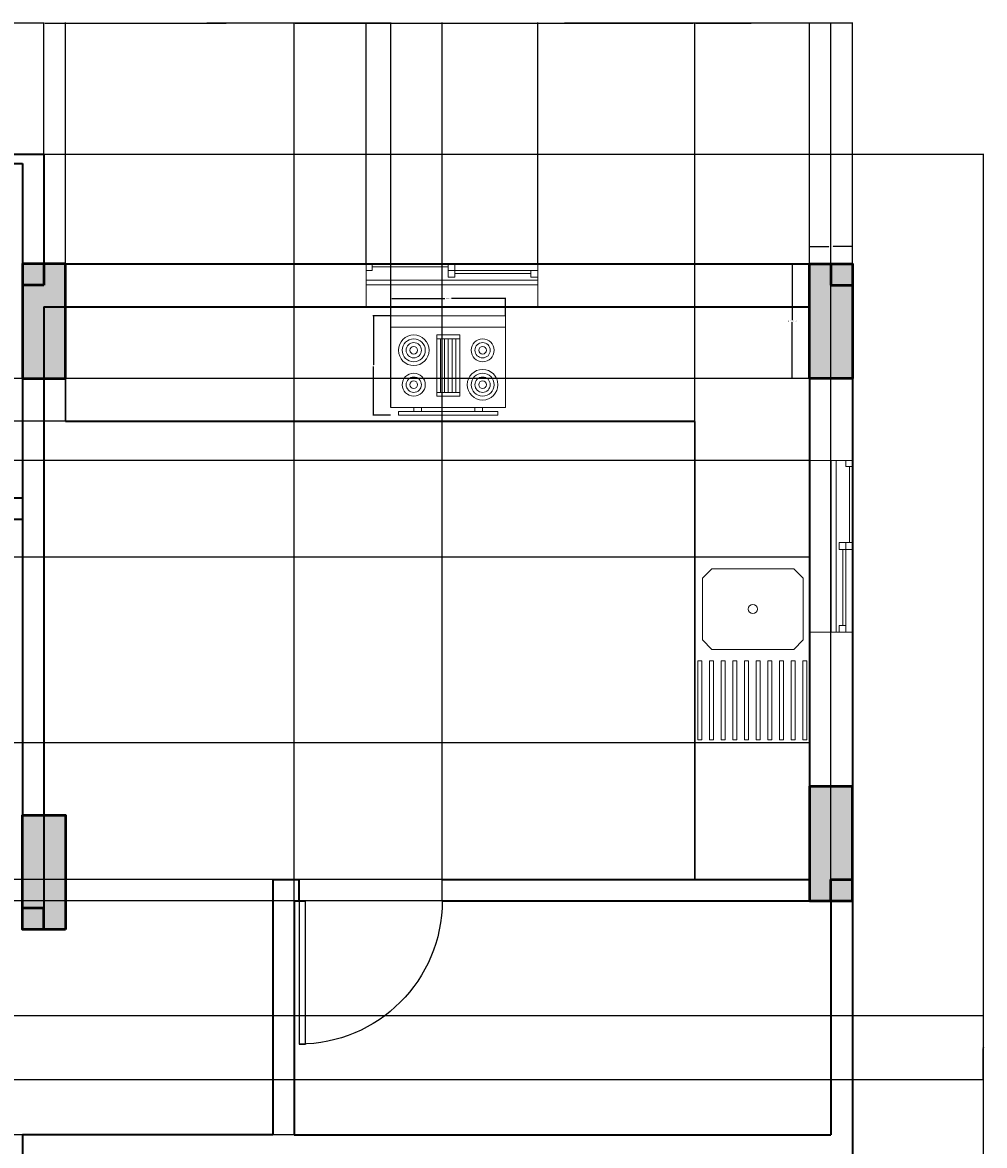
# Model space of a CAD drawing. Units: inches. Extents: x 393 to 993, y 153 to 660.
# Tile 6 of 6: x 791 to 993, y 425 to 660. Entities that reach past the tile are written whole.
import ezdxf

# ---------------------------------------------------------------- set-up
doc = ezdxf.new("R2010")
doc.units = ezdxf.units.IN
doc.header["$MEASUREMENT"] = 0
for name, color, linetype, lineweight in [('A-ANNO-DIMS', 2, 'Continuous', 18), ('A-COLS', 40, 'Continuous', 50), ('A-EQPM', 8, 'Continuous', 18), ('A-FLOR-CASE', 72, 'Continuous', 25), ('A-FLOR-FIXT', 9, 'Continuous', 18), ('A-GLAZ', 4, 'Continuous', 20), ('A-WALL', 40, 'Continuous', 35), ('DOORS', 32, 'Continuous', 25)]:
    doc.layers.add(name, color=color, linetype=linetype, lineweight=lineweight)
doc.styles.get("Standard").update_dxf_attribs({"font": 'arial.ttf'})
doc.dimstyles.get("Standard").update_dxf_attribs({"dimtxt": 0.18, "dimasz": 0.18, "dimexe": 0.18, "dimexo": 0.0625, "dimgap": 0.09, "dimtad": 0, "dimtih": 1, "dimtoh": 1, "dimdec": 1, "dimzin": 0, "dimdsep": 46, "dimlunit": 3, "dimtxsty": 'Standard', "dimcen": 0.09, "dimadec": 0, "dimazin": 0, "dimtfac": 1, "dimtdec": 1, "dimtofl": 0, "dimtmove": 0, "dimatfit": 3, "dimfxl": 1, "dimtolj": 1, "dimtzin": 0, "dimarcsym": 0})

# ---------------------------------------------------------------- blocks, each defined once
blk = doc.blocks.new('*U3')
for p, q in [((0, 0), (0, -6)), ((40, 0), (40, -6))]:
    blk.add_line(p, q)
blk.add_lwpolyline([(0, 0), (0, 40), (1.75, 40), (1.75, 0)], close=True)
blk.add_arc((0, 0), 40, 0, 90)
blk = doc.blocks.new('W')
for p, q in [((518.15, 606.48), (554.15, 606.48)), ((518.15, 605.48), (554.15, 605.48))]:
    blk.add_line(p, q)
for points in [[(518.15, 609.91), (554.15, 609.91), (554.15, 600.91), (518.15, 600.91)], [(519.42, 609.91), (518.15, 609.91), (518.15, 608.51), (519.42, 608.51)], [(519.42, 609.91), (535.35, 609.91), (535.35, 609.3), (519.42, 609.3)], [(535.35, 609.91), (536.78, 609.91), (536.78, 608.51), (535.35, 608.51)], [(536.78, 608.51), (535.35, 608.51), (535.35, 607.12), (536.78, 607.12)], [(552.72, 608.51), (536.78, 608.51), (536.78, 607.91), (552.72, 607.91)], [(552.72, 608.51), (554.15, 608.51), (554.15, 607.12), (552.72, 607.12)]]:
    blk.add_lwpolyline(points, close=True)
blk = doc.blocks.new('Range-Oven - 30 in top')
for p, q in [((0, -3), (30, -3)), ((12, -6), (18, -6)), ((13, -20), (13, -6)), ((14, -6), (14, -20)), ((15, -20), (15, -6)), ((16, -6), (16, -20)), ((17, -20), (17, -6)), ((18, -20), (12, -20)), ((6, -24), (6, -25)), ((8, -25), (8, -24)), ((22, -25), (22, -24)), ((24, -24), (24, -25))]:
    blk.add_line(p, q)
for points in [[(0, -24), (0, 0), (30, 0), (30, -24)], [(12, -21), (12, -5), (18, -5), (18, -21)], [(2, -26), (2, -25), (28, -25), (28, -26)]]:
    blk.add_lwpolyline(points, close=True)
for centre, radius in [((6, -9), 4), ((6, -9), 3), ((6, -9), 2), ((6, -9), 1), ((24, -9), 3), ((24, -9), 2), ((24, -9), 1), ((24, -18), 4), ((6, -18), 3), ((6, -18), 2), ((6, -18), 1), ((24, -18), 3), ((24, -18), 2), ((24, -18), 1)]:
    blk.add_circle(centre, radius)
blk = doc.blocks.new('COL-9X24-RH')
h = blk.add_hatch(color=256)
h.dxf.hatch_style = 1
h.paths.add_polyline_path([(4.5, 19.5), (4.5, 24), (0, 24), (0, 0), (9, 0), (9, 19.5)])
h = blk.add_hatch(color=256)
h.dxf.hatch_style = 1
h.paths.add_polyline_path([(4.5, 19.5), (9, 19.5), (9, 24), (4.5, 24)])
for p, q in [((4.5, 24), (4.5, 19.5)), ((4.5, 24), (9, 24)), ((9, 24), (9, 19.5)), ((4.5, 19.5), (9, 19.5))]:
    blk.add_line(p, q)
blk.add_lwpolyline([(0, 24), (9, 24), (9, 0), (0, 0), (0, 24)])
blk = doc.blocks.new('COL-9X24-LH')
h = blk.add_hatch(color=256)
h.dxf.hatch_style = 1
h.paths.add_polyline_path([(4.5, 24), (0, 24), (0, 19.5), (4.5, 19.5)])
h = blk.add_hatch(color=256)
h.dxf.hatch_style = 1
h.paths.add_polyline_path([(4.5, 19.5), (0, 19.5), (0, 0), (9, 0), (9, 24), (4.5, 24)])
for p, q in [((4.5, 24), (0, 24)), ((0, 24), (0, 19.5)), ((4.5, 24), (4.5, 19.5)), ((4.5, 19.5), (0, 19.5))]:
    blk.add_line(p, q)
blk.add_lwpolyline([(9, 24), (0, 24), (0, 0), (9, 0), (9, 24)])
blk = doc.blocks.new('*D18')
at = {"layer": 'A-ANNO-DIMS', "color": 0, "lineweight": -2, "transparency": 16777216}
for p, q in [((956.42, 609.91), (952.7, 609.91)), ((952.88, 609.73), (952.88, 598.09)), ((952.88, 586.09), (952.88, 597.72)), ((956.42, 585.91), (952.7, 585.91))]:
    blk.add_line(p, q, dxfattribs=at)
at = {"layer": 'A-ANNO-DIMS', "color": 0, "transparency": 16777216}
for points in [[(952.85, 609.73), (952.91, 609.73), (952.88, 609.91)], [(952.85, 586.09), (952.91, 586.09), (952.88, 585.91)]]:
    blk.add_solid(points, dxfattribs=at)
at = {"layer": 'Defpoints', "color": 0, "transparency": 16777216}
for p in [(952.88, 609.91), (956.48, 609.91), (956.48, 585.91)]:
    blk.add_point(p, dxfattribs=at)
at = {"layer": 'A-ANNO-DIMS', "color": 0, "transparency": 16777216, "insert": (952.88, 597.91), "char_height": 0.18, "attachment_point": 5}
blk.add_mtext('\\A1;RH COL. 24 TYP.', dxfattribs=at)
blk = doc.blocks.new('*D19')
at = {"layer": 'A-ANNO-DIMS', "color": 0, "lineweight": -2, "transparency": 16777216}
for p, q in [((956.48, 609.97), (956.48, 613.69)), ((956.66, 613.51), (960.52, 613.51)), ((965.3, 613.51), (961.44, 613.51)), ((965.48, 609.97), (965.48, 613.69))]:
    blk.add_line(p, q, dxfattribs=at)
at = {"layer": 'A-ANNO-DIMS', "color": 0, "transparency": 16777216}
for points in [[(956.66, 613.54), (956.66, 613.48), (956.48, 613.51)], [(965.3, 613.54), (965.3, 613.48), (965.48, 613.51)]]:
    blk.add_solid(points, dxfattribs=at)
at = {"layer": 'Defpoints', "color": 0, "transparency": 16777216}
for p in [(965.48, 613.51), (956.48, 609.91), (965.48, 609.91)]:
    blk.add_point(p, dxfattribs=at)
at = {"layer": 'A-ANNO-DIMS', "color": 0, "transparency": 16777216, "insert": (960.98, 613.51), "char_height": 0.18, "attachment_point": 5}
blk.add_mtext('\\A1;9 TYP.', dxfattribs=at)
blk = doc.blocks.new('*D42')
at = {"layer": 'A-ANNO-DIMS', "color": 0, "lineweight": -2, "transparency": 16777216}
for p, q in [((868.71, 599.08), (868.71, 602.8)), ((868.89, 602.62), (880.04, 602.62)), ((892.59, 602.62), (881.43, 602.62)), ((892.77, 599.08), (892.77, 602.8))]:
    blk.add_line(p, q, dxfattribs=at)
at = {"layer": 'A-ANNO-DIMS', "color": 0, "transparency": 16777216}
for points in [[(868.89, 602.65), (868.89, 602.59), (868.71, 602.62)], [(892.59, 602.65), (892.59, 602.59), (892.77, 602.62)]]:
    blk.add_solid(points, dxfattribs=at)
at = {"layer": 'Defpoints', "color": 0, "transparency": 16777216}
for p in [(892.77, 602.62), (868.71, 599.02), (892.77, 599.02)]:
    blk.add_point(p, dxfattribs=at)
at = {"layer": 'A-ANNO-DIMS', "color": 0, "transparency": 16777216, "insert": (880.74, 602.62), "char_height": 0.18, "attachment_point": 5}
blk.add_mtext('\\A1;RANGE 24', dxfattribs=at)
blk = doc.blocks.new('*D43')
at = {"layer": 'A-ANNO-DIMS', "color": 0, "lineweight": -2, "transparency": 16777216}
for p, q in [((868.65, 599.02), (864.92, 599.02)), ((865.1, 598.84), (865.1, 588.77)), ((865.1, 578.35), (865.1, 588.41)), ((868.65, 578.17), (864.92, 578.17))]:
    blk.add_line(p, q, dxfattribs=at)
at = {"layer": 'A-ANNO-DIMS', "color": 0, "transparency": 16777216}
for points in [[(865.07, 598.84), (865.13, 598.84), (865.1, 599.02)], [(865.07, 578.35), (865.13, 578.35), (865.1, 578.17)]]:
    blk.add_solid(points, dxfattribs=at)
at = {"layer": 'Defpoints', "color": 0, "transparency": 16777216}
for p in [(865.1, 599.02), (868.71, 599.02), (868.71, 578.17)]:
    blk.add_point(p, dxfattribs=at)
at = {"layer": 'A-ANNO-DIMS', "color": 0, "transparency": 16777216, "insert": (865.1, 588.59), "char_height": 0.18, "attachment_point": 5}
blk.add_mtext('\\A1;21', dxfattribs=at)
blk = doc.blocks.new('*D45')
at = {"layer": 'A-ANNO-DIMS', "color": 0, "lineweight": -2, "transparency": 16777216}
for p, q in [((796.04, 632.91), (993.06, 632.91)), ((992.88, 632.73), (992.88, 407.09)), ((992.88, 181.09), (992.88, 406.72)), ((965.54, 180.91), (993.06, 180.91))]:
    blk.add_line(p, q, dxfattribs=at)
at = {"layer": 'A-ANNO-DIMS', "color": 0, "transparency": 16777216}
for points in [[(992.85, 632.73), (992.91, 632.73), (992.88, 632.91)], [(992.85, 181.09), (992.91, 181.09), (992.88, 180.91)]]:
    blk.add_solid(points, dxfattribs=at)
at = {"layer": 'Defpoints', "color": 0, "transparency": 16777216}
for p in [(795.98, 632.91), (992.88, 632.91), (965.48, 180.91)]:
    blk.add_point(p, dxfattribs=at)
at = {"layer": 'A-ANNO-DIMS', "color": 0, "transparency": 16777216, "insert": (992.88, 406.91), "char_height": 0.18, "attachment_point": 5}
blk.add_mtext('\\A1;452', dxfattribs=at)
blk = doc.blocks.new('*D48')
at = {"layer": 'A-ANNO-DIMS', "color": 0, "lineweight": -2, "transparency": 16777216}
for p, q in [((642.98, 632.97), (642.98, 660.49)), ((643.16, 660.31), (719.2, 660.31)), ((795.8, 660.31), (719.76, 660.31)), ((795.98, 632.97), (795.98, 660.49))]:
    blk.add_line(p, q, dxfattribs=at)
at = {"layer": 'A-ANNO-DIMS', "color": 0, "transparency": 16777216}
for points in [[(643.16, 660.34), (643.16, 660.28), (642.98, 660.31)], [(795.8, 660.34), (795.8, 660.28), (795.98, 660.31)]]:
    blk.add_solid(points, dxfattribs=at)
at = {"layer": 'Defpoints', "color": 0, "transparency": 16777216}
for p in [(795.98, 660.31), (642.98, 632.91), (795.98, 632.91)]:
    blk.add_point(p, dxfattribs=at)
at = {"layer": 'A-ANNO-DIMS', "color": 0, "transparency": 16777216, "insert": (719.48, 660.31), "char_height": 0.18, "attachment_point": 5}
blk.add_mtext('\\A1;153', dxfattribs=at)
blk = doc.blocks.new('*D49')
at = {"layer": 'A-ANNO-DIMS', "color": 0, "lineweight": -2, "transparency": 16777216}
for p, q in [((795.98, 609.97), (795.98, 660.49)), ((796.16, 660.31), (829.36, 660.31)), ((863.34, 660.31), (830.15, 660.31)), ((863.52, 609.97), (863.52, 660.49))]:
    blk.add_line(p, q, dxfattribs=at)
at = {"layer": 'A-ANNO-DIMS', "color": 0, "transparency": 16777216}
for points in [[(796.16, 660.34), (796.16, 660.28), (795.98, 660.31)], [(863.34, 660.34), (863.34, 660.28), (863.52, 660.31)]]:
    blk.add_solid(points, dxfattribs=at)
at = {"layer": 'Defpoints', "color": 0, "transparency": 16777216}
for p in [(863.52, 660.31), (795.98, 609.91), (863.52, 609.91)]:
    blk.add_point(p, dxfattribs=at)
at = {"layer": 'A-ANNO-DIMS', "color": 0, "transparency": 16777216, "insert": (829.75, 660.31), "char_height": 0.18, "attachment_point": 5}
blk.add_mtext('\\A1;67.54', dxfattribs=at)
blk = doc.blocks.new('*D50')
at = {"layer": 'A-ANNO-DIMS', "color": 0, "lineweight": -2, "transparency": 16777216}
for p, q in [((899.52, 609.97), (899.52, 660.49)), ((899.7, 660.31), (932.11, 660.31)), ((965.3, 660.31), (932.9, 660.31)), ((965.48, 609.97), (965.48, 660.49))]:
    blk.add_line(p, q, dxfattribs=at)
at = {"layer": 'A-ANNO-DIMS', "color": 0, "transparency": 16777216}
for points in [[(899.7, 660.34), (899.7, 660.28), (899.52, 660.31)], [(965.3, 660.34), (965.3, 660.28), (965.48, 660.31)]]:
    blk.add_solid(points, dxfattribs=at)
at = {"layer": 'Defpoints', "color": 0, "transparency": 16777216}
for p in [(965.48, 660.31), (899.52, 609.91), (965.48, 609.91)]:
    blk.add_point(p, dxfattribs=at)
at = {"layer": 'A-ANNO-DIMS', "color": 0, "transparency": 16777216, "insert": (932.5, 660.31), "char_height": 0.18, "attachment_point": 5}
blk.add_mtext('\\A1;65.96', dxfattribs=at)
blk = doc.blocks.new('*D57')
at = {"layer": 'A-ANNO-DIMS', "color": 0, "lineweight": -2, "transparency": 16777216}
for p, q in [((848.48, 427.47), (848.48, 660.49)), ((848.66, 660.31), (904.34, 660.31)), ((960.8, 660.31), (905.12, 660.31)), ((960.98, 427.47), (960.98, 660.49))]:
    blk.add_line(p, q, dxfattribs=at)
at = {"layer": 'A-ANNO-DIMS', "color": 0, "transparency": 16777216}
for points in [[(848.66, 660.34), (848.66, 660.28), (848.48, 660.31)], [(960.8, 660.34), (960.8, 660.28), (960.98, 660.31)]]:
    blk.add_solid(points, dxfattribs=at)
at = {"layer": 'Defpoints', "color": 0, "transparency": 16777216}
for p in [(960.98, 660.31), (848.48, 427.41), (960.98, 427.41)]:
    blk.add_point(p, dxfattribs=at)
at = {"layer": 'A-ANNO-DIMS', "color": 0, "transparency": 16777216, "insert": (904.73, 660.31), "char_height": 0.18, "attachment_point": 5}
blk.add_mtext('\\A1;112.5', dxfattribs=at)
blk = doc.blocks.new('*D58')
at = {"layer": 'A-ANNO-DIMS', "color": 0, "lineweight": -2, "transparency": 16777216}
for p, q in [((932.48, 480.97), (932.48, 660.49)), ((932.66, 660.31), (944.26, 660.31)), ((956.3, 660.31), (944.7, 660.31)), ((956.48, 480.97), (956.48, 660.49))]:
    blk.add_line(p, q, dxfattribs=at)
at = {"layer": 'A-ANNO-DIMS', "color": 0, "transparency": 16777216}
for points in [[(932.66, 660.34), (932.66, 660.28), (932.48, 660.31)], [(956.3, 660.34), (956.3, 660.28), (956.48, 660.31)]]:
    blk.add_solid(points, dxfattribs=at)
at = {"layer": 'Defpoints', "color": 0, "transparency": 16777216}
for p in [(956.48, 660.31), (932.48, 480.91), (956.48, 480.91)]:
    blk.add_point(p, dxfattribs=at)
at = {"layer": 'A-ANNO-DIMS', "color": 0, "transparency": 16777216, "insert": (944.48, 660.31), "char_height": 0.18, "attachment_point": 5}
blk.add_mtext('\\A1;24', dxfattribs=at)
blk = doc.blocks.new('*D63')
at = {"layer": 'A-ANNO-DIMS', "color": 0, "lineweight": -2, "transparency": 16777216}
for p, q in [((960.92, 476.41), (393.4, 476.41)), ((393.58, 476.23), (393.58, 452.09)), ((393.58, 427.59), (393.58, 451.72)), ((960.92, 427.41), (393.4, 427.41))]:
    blk.add_line(p, q, dxfattribs=at)
at = {"layer": 'A-ANNO-DIMS', "color": 0, "transparency": 16777216}
for points in [[(393.55, 476.23), (393.61, 476.23), (393.58, 476.41)], [(393.55, 427.59), (393.61, 427.59), (393.58, 427.41)]]:
    blk.add_solid(points, dxfattribs=at)
at = {"layer": 'Defpoints', "color": 0, "transparency": 16777216}
for p in [(393.58, 476.41), (960.98, 476.41), (960.98, 427.41)]:
    blk.add_point(p, dxfattribs=at)
at = {"layer": 'A-ANNO-DIMS', "color": 0, "transparency": 16777216, "insert": (393.58, 451.91), "char_height": 0.18, "attachment_point": 5}
blk.add_mtext('\\A1;49', dxfattribs=at)
blk = doc.blocks.new('*D64')
at = {"layer": 'A-ANNO-DIMS', "color": 0, "lineweight": -2, "transparency": 16777216}
for p, q in [((932.42, 576.91), (393.4, 576.91)), ((393.58, 576.73), (393.58, 529.09)), ((393.58, 481.09), (393.58, 528.72)), ((932.42, 480.91), (393.4, 480.91))]:
    blk.add_line(p, q, dxfattribs=at)
at = {"layer": 'A-ANNO-DIMS', "color": 0, "transparency": 16777216}
for points in [[(393.55, 576.73), (393.61, 576.73), (393.58, 576.91)], [(393.55, 481.09), (393.61, 481.09), (393.58, 480.91)]]:
    blk.add_solid(points, dxfattribs=at)
at = {"layer": 'Defpoints', "color": 0, "transparency": 16777216}
for p in [(393.58, 576.91), (932.48, 576.91), (932.48, 480.91)]:
    blk.add_point(p, dxfattribs=at)
at = {"layer": 'A-ANNO-DIMS', "color": 0, "transparency": 16777216, "insert": (393.58, 528.91), "char_height": 0.18, "attachment_point": 5}
blk.add_mtext('\\A1;96', dxfattribs=at)
blk = doc.blocks.new('*D72')
at = {"layer": 'A-ANNO-DIMS', "color": 0, "lineweight": -2, "transparency": 16777216}
for p, q in [((481.04, 452.41), (993.06, 452.41)), ((992.88, 452.23), (992.88, 445.86)), ((992.88, 439.14), (992.88, 445.5)), ((481.04, 438.96), (993.06, 438.96))]:
    blk.add_line(p, q, dxfattribs=at)
at = {"layer": 'A-ANNO-DIMS', "color": 0, "transparency": 16777216}
for points in [[(992.85, 452.23), (992.91, 452.23), (992.88, 452.41)], [(992.85, 439.14), (992.91, 439.14), (992.88, 438.96)]]:
    blk.add_solid(points, dxfattribs=at)
at = {"layer": 'Defpoints', "color": 0, "transparency": 16777216}
for p in [(480.98, 452.41), (992.88, 452.41), (480.98, 438.96)]:
    blk.add_point(p, dxfattribs=at)
at = {"layer": 'A-ANNO-DIMS', "color": 0, "transparency": 16777216, "insert": (992.88, 445.68), "char_height": 0.18, "attachment_point": 5}
blk.add_mtext('\\A1;13.45', dxfattribs=at)
blk = doc.blocks.new('*D74')
at = {"layer": 'A-ANNO-DIMS', "color": 0, "lineweight": -2, "transparency": 16777216}
for p, q in [((956.42, 585.91), (393.4, 585.91)), ((393.58, 585.73), (393.58, 577.48)), ((393.58, 568.88), (393.58, 577.12)), ((956.42, 568.7), (393.4, 568.7))]:
    blk.add_line(p, q, dxfattribs=at)
at = {"layer": 'A-ANNO-DIMS', "color": 0, "transparency": 16777216}
for points in [[(393.55, 585.73), (393.61, 585.73), (393.58, 585.91)], [(393.55, 568.88), (393.61, 568.88), (393.58, 568.7)]]:
    blk.add_solid(points, dxfattribs=at)
at = {"layer": 'Defpoints', "color": 0, "transparency": 16777216}
for p in [(393.58, 585.91), (956.48, 585.91), (956.48, 568.7)]:
    blk.add_point(p, dxfattribs=at)
at = {"layer": 'A-ANNO-DIMS', "color": 0, "transparency": 16777216, "insert": (393.58, 577.3), "char_height": 0.18, "attachment_point": 5}
blk.add_mtext('\\A1;17.21', dxfattribs=at)
blk = doc.blocks.new('*D78')
at = {"layer": 'A-ANNO-DIMS', "color": 0, "lineweight": -2, "transparency": 16777216}
for p, q in [((879.48, 480.97), (879.48, 660.49)), ((879.66, 660.31), (905.76, 660.31)), ((932.3, 660.31), (906.2, 660.31)), ((932.48, 480.97), (932.48, 660.49))]:
    blk.add_line(p, q, dxfattribs=at)
at = {"layer": 'A-ANNO-DIMS', "color": 0, "transparency": 16777216}
for points in [[(879.66, 660.34), (879.66, 660.28), (879.48, 660.31)], [(932.3, 660.34), (932.3, 660.28), (932.48, 660.31)]]:
    blk.add_solid(points, dxfattribs=at)
at = {"layer": 'Defpoints', "color": 0, "transparency": 16777216}
for p in [(932.48, 660.31), (879.48, 480.91), (932.48, 480.91)]:
    blk.add_point(p, dxfattribs=at)
at = {"layer": 'A-ANNO-DIMS', "color": 0, "transparency": 16777216, "insert": (905.98, 660.31), "char_height": 0.18, "attachment_point": 5}
blk.add_mtext('\\A1;53', dxfattribs=at)
blk = doc.blocks.new('*D80')
at = {"layer": 'A-ANNO-DIMS', "color": 0, "lineweight": -2, "transparency": 16777216}
for p, q in [((879.42, 480.91), (393.4, 480.91)), ((393.58, 480.73), (393.58, 478.84)), ((393.58, 476.59), (393.58, 478.48)), ((879.42, 476.41), (393.4, 476.41))]:
    blk.add_line(p, q, dxfattribs=at)
at = {"layer": 'A-ANNO-DIMS', "color": 0, "transparency": 16777216}
for points in [[(393.55, 480.73), (393.61, 480.73), (393.58, 480.91)], [(393.55, 476.59), (393.61, 476.59), (393.58, 476.41)]]:
    blk.add_solid(points, dxfattribs=at)
at = {"layer": 'Defpoints', "color": 0, "transparency": 16777216}
for p in [(393.58, 480.91), (879.48, 480.91), (879.48, 476.41)]:
    blk.add_point(p, dxfattribs=at)
at = {"layer": 'A-ANNO-DIMS', "color": 0, "transparency": 16777216, "insert": (393.58, 478.66), "char_height": 0.18, "attachment_point": 5}
blk.add_mtext('\\A1;4.5', dxfattribs=at)
blk = doc.blocks.new('*D82')
at = {"layer": 'A-ANNO-DIMS', "color": 0, "lineweight": -2, "transparency": 16777216}
for p, q in [((800.48, 576.97), (800.48, 660.49)), ((800.66, 660.31), (834.2, 660.31)), ((868.53, 660.31), (834.99, 660.31)), ((868.71, 579.83), (868.71, 660.49))]:
    blk.add_line(p, q, dxfattribs=at)
at = {"layer": 'A-ANNO-DIMS', "color": 0, "transparency": 16777216}
for points in [[(800.66, 660.34), (800.66, 660.28), (800.48, 660.31)], [(868.53, 660.34), (868.53, 660.28), (868.71, 660.31)]]:
    blk.add_solid(points, dxfattribs=at)
at = {"layer": 'Defpoints', "color": 0, "transparency": 16777216}
for p in [(868.71, 660.31), (868.71, 579.77), (800.48, 576.91)]:
    blk.add_point(p, dxfattribs=at)
at = {"layer": 'A-ANNO-DIMS', "color": 0, "transparency": 16777216, "insert": (834.6, 660.31), "char_height": 0.18, "attachment_point": 5}
blk.add_mtext('\\A1;68.23', dxfattribs=at)
blk = doc.blocks.new('*D84')
at = {"layer": 'A-ANNO-DIMS', "color": 0, "lineweight": -2, "transparency": 16777216}
for p, q in [((956.42, 548.43), (393.4, 548.43)), ((393.58, 548.25), (393.58, 529.18)), ((393.58, 509.74), (393.58, 528.81)), ((956.42, 509.56), (393.4, 509.56))]:
    blk.add_line(p, q, dxfattribs=at)
at = {"layer": 'A-ANNO-DIMS', "color": 0, "transparency": 16777216}
for points in [[(393.55, 548.25), (393.61, 548.25), (393.58, 548.43)], [(393.55, 509.74), (393.61, 509.74), (393.58, 509.56)]]:
    blk.add_solid(points, dxfattribs=at)
at = {"layer": 'Defpoints', "color": 0, "transparency": 16777216}
for p in [(393.58, 548.43), (956.48, 548.43), (956.48, 509.56)]:
    blk.add_point(p, dxfattribs=at)
at = {"layer": 'A-ANNO-DIMS', "color": 0, "transparency": 16777216, "insert": (393.58, 529), "char_height": 0.18, "attachment_point": 5}
blk.add_mtext('\\A1;38.87', dxfattribs=at)

msp = doc.modelspace()

# ---------------------------------------------------------------- linework, layer by layer
at = {"layer": 'A-FLOR-CASE'}
for p, q in [((800.4798, 600.9066), (800.4798, 576.9066)), ((800.4798, 576.9066), (932.4798, 576.9066)), ((932.4798, 576.9066), (932.4798, 480.9066))]:
    msp.add_line(p, q, dxfattribs=at)
at = {"layer": 'A-FLOR-FIXT'}
for points in [[(932.4798, 548.43), (956.4798, 548.43), (956.4798, 509.5613), (932.4798, 509.5613)], [(936.0192, 546.0319), (953.1906, 546.0319), (955.1906, 544.0319), (955.1906, 531.1242), (953.1906, 529.1242), (936.0192, 529.1242), (934.0192, 531.1242), (934.0192, 544.0319)], [(933.0558, 526.7467), (933.9083, 526.7467), (933.9083, 510.1556), (933.0558, 510.1556)], [(935.5054, 526.7467), (936.3578, 526.7467), (936.3578, 510.1556), (935.5054, 510.1556)], [(937.955, 526.7467), (938.8074, 526.7467), (938.8074, 510.1556), (937.955, 510.1556)], [(940.4046, 526.7467), (941.257, 526.7467), (941.257, 510.1556), (940.4046, 510.1556)], [(942.8542, 526.7467), (943.7066, 526.7467), (943.7066, 510.1556), (942.8542, 510.1556)], [(945.3038, 526.7467), (946.1562, 526.7467), (946.1562, 510.1556), (945.3038, 510.1556)], [(947.7534, 526.7467), (948.6058, 526.7467), (948.6058, 510.1556), (947.7534, 510.1556)], [(950.203, 526.7467), (951.0554, 526.7467), (951.0554, 510.1556), (950.203, 510.1556)], [(952.6526, 526.7467), (953.505, 526.7467), (953.505, 510.1556), (952.6526, 510.1556)], [(955.1021, 526.7467), (955.9546, 526.7467), (955.9546, 510.1556), (955.1021, 510.1556)]]:
    msp.add_lwpolyline(points, close=True, dxfattribs=at)
msp.add_circle((944.6049, 537.578), 0.9726, dxfattribs=at)
at = {"layer": 'A-WALL'}
for p, q in [((642.9798, 632.9066), (795.9798, 632.9066)), ((647.4798, 630.9066), (791.4798, 630.9066)), ((791.4798, 630.9066), (791.4798, 470.4066)), ((795.9798, 632.9066), (795.9798, 609.9066)), ((795.9798, 609.9066), (965.4798, 609.9066)), ((965.4798, 609.9066), (965.4798, 180.9066)), ((795.9798, 600.9066), (956.4798, 600.9066)), ((795.9798, 600.9066), (795.9798, 470.4066)), ((956.4798, 600.9066), (956.4798, 480.9066)), ((647.4798, 560.9066), (791.4798, 560.9066)), ((647.4798, 556.4066), (791.4798, 556.4066)), ((843.9798, 480.9066), (849.4798, 480.9066)), ((843.9798, 480.9066), (843.9798, 427.4066)), ((849.4798, 476.4066), (849.4798, 480.9066)), ((879.4798, 480.9066), (956.4798, 480.9066)), ((848.4798, 476.4066), (850.7923, 476.4066)), ((848.4798, 476.4066), (848.4798, 427.4066)), ((848.4798, 476.4066), (849.4798, 476.4066)), ((879.4798, 476.4066), (956.4798, 476.4066)), ((960.9798, 476.4066), (960.9798, 427.4066)), ((843.9798, 427.4066), (791.4798, 427.4066)), ((791.4798, 427.4066), (791.4798, 362.9066)), ((848.4798, 427.4066), (960.9798, 427.4066))]:
    msp.add_line(p, q, dxfattribs=at)

# ---------------------------------------------------------------- block references
at = {"layer": 'A-COLS'}
for name, p in [('COL-9X24-LH', (791.48, 585.907)), ('COL-9X24-RH', (956.48, 585.907))]:
    msp.add_blockref(name, p, dxfattribs=at)
at = {"layer": 'A-COLS', "rotation": 180}
for name, p in [('COL-9X24-LH', (965.4796, 500.4063)), ('COL-9X24-RH', (800.4796, 494.4063))]:
    msp.add_blockref(name, p, dxfattribs=at)
at = {"layer": 'A-EQPM', "xscale": 0.8018281955840633, "yscale": 0.8018281955840633, "zscale": 0.8018281955840633}
msp.add_blockref('Range-Oven - 30 in top', (868.7106, 599.0163), dxfattribs=at)
at = {"layer": 'A-GLAZ'}
msp.add_blockref('W', (345.3756, 0), dxfattribs=at)
at = {"layer": 'A-GLAZ', "rotation": 270}
msp.add_blockref('W', (355.5732, 1086.8471), dxfattribs=at)
at = {"layer": 'DOORS', "xscale": -0.75, "yscale": 0.75, "zscale": 0.75, "rotation": 180}
msp.add_blockref('*U3', (849.4798, 476.4066), dxfattribs=at)

# ---------------------------------------------------------------- dimensions: what is measured, and where the dimension line sits
at = {"layer": 'A-ANNO-DIMS'}
for base, p1, p2, override, picture, middle in [((795.9798, 660.3066), (642.9798, 632.9066), (795.9798, 632.9066), {"dimdec": 0, "dimlfac": 1, "dimrnd": 0, "dimzin": 0, "dimdsep": 46, "dimlunit": 2}, '*D48', (719.4798, 660.3066)), ((863.5243, 660.3066), (795.9798, 609.9066), (863.5243, 609.9066), {"dimdec": 2, "dimlfac": 1, "dimrnd": 0, "dimzin": 0, "dimdsep": 46, "dimlunit": 2}, '*D49', (829.7521, 660.3066)), ((868.7106, 660.3066), (800.4798, 576.9066), (868.7106, 579.7724), {"dimdec": 2, "dimlfac": 1, "dimrnd": 0, "dimzin": 0, "dimdsep": 46, "dimlunit": 2}, '*D82', (834.5952, 660.3066)), ((960.9798, 660.3066), (848.4798, 427.4066), (960.9798, 427.4066), {"dimdec": 1, "dimlfac": 1, "dimrnd": 0, "dimzin": 0, "dimdsep": 46, "dimlunit": 2}, '*D57', (904.7298, 660.3066)), ((932.4798, 660.3066), (879.4798, 480.9066), (932.4798, 480.9066), {"dimdec": 0, "dimlfac": 1, "dimrnd": 0, "dimzin": 0, "dimdsep": 46, "dimlunit": 2}, '*D78', (905.9798, 660.3066)), ((965.4798, 660.3066), (899.5243, 609.9066), (965.4798, 609.9066), {"dimdec": 2, "dimlfac": 1, "dimrnd": 0, "dimzin": 0, "dimdsep": 46, "dimlunit": 2}, '*D50', (932.5021, 660.3066)), ((956.4798, 660.3066), (932.4798, 480.9066), (956.4798, 480.9066), {"dimdec": 0, "dimlfac": 1, "dimrnd": 0, "dimzin": 0, "dimdsep": 46, "dimlunit": 2}, '*D58', (944.4798, 660.3066))]:
    dim = msp.add_linear_dim(base=base, p1=p1, p2=p2, dimstyle='Standard', override=override, dxfattribs=at)
    dim.commit()
    dim.dimension.update_dxf_attribs({"geometry": picture, "text_midpoint": middle})
for base, p1, p2, override, picture, middle in [((992.8798, 632.9066), (965.4798, 180.9066), (795.9798, 632.9066), {"dimdec": 0, "dimlfac": 1, "dimrnd": 0, "dimzin": 0, "dimdsep": 46, "dimlunit": 2}, '*D45', (992.8798, 406.9066)), ((865.1024, 599.0163), (868.7106, 578.1688), (868.7106, 599.0163), {"dimdec": 0, "dimlfac": 1, "dimrnd": 0, "dimzin": 0, "dimdsep": 46, "dimlunit": 2}, '*D43', (865.1024, 588.5926)), ((393.5798, 585.9066), (956.4798, 568.6983), (956.4798, 585.9066), {"dimdec": 2, "dimlfac": 1, "dimrnd": 0, "dimzin": 0, "dimdsep": 46, "dimlunit": 2}, '*D74', (393.5798, 577.3025)), ((393.5798, 576.9066), (932.4798, 480.9066), (932.4798, 576.9066), {"dimdec": 0, "dimlfac": 1, "dimrnd": 0, "dimzin": 0, "dimdsep": 46, "dimlunit": 2}, '*D64', (393.5798, 528.9066)), ((393.5798, 548.43), (956.4798, 509.5613), (956.4798, 548.43), {"dimdec": 2, "dimlfac": 1, "dimrnd": 0, "dimzin": 0, "dimdsep": 46, "dimlunit": 2}, '*D84', (393.5798, 528.9957)), ((393.5798, 480.9066), (879.4798, 476.4066), (879.4798, 480.9066), {"dimdec": 1, "dimlfac": 1, "dimrnd": 0, "dimzin": 0, "dimdsep": 46, "dimlunit": 2}, '*D80', (393.5798, 478.6566)), ((393.5798, 476.4066), (960.9798, 427.4066), (960.9798, 476.4066), {"dimdec": 0, "dimlfac": 1, "dimrnd": 0, "dimzin": 0, "dimdsep": 46, "dimlunit": 2}, '*D63', (393.5798, 451.9066)), ((992.8798, 452.4066), (480.9798, 438.9566), (480.9798, 452.4066), {"dimdec": 2, "dimlfac": 1, "dimrnd": 0, "dimzin": 0, "dimdsep": 46, "dimlunit": 2}, '*D72', (992.8798, 445.6816))]:
    dim = msp.add_linear_dim(base=base, p1=p1, p2=p2, angle=90, dimstyle='Standard', override=override, dxfattribs=at)
    dim.commit()
    dim.dimension.update_dxf_attribs({"geometry": picture, "text_midpoint": middle})
for base, p1, p2, text, picture, middle in [((965.4798, 613.5066), (956.4798, 609.9066), (965.4798, 609.9066), '<> TYP.', '*D19', (960.9798, 613.5066)), ((892.7655, 602.6245), (868.7106, 599.0163), (892.7655, 599.0163), 'RANGE <>', '*D42', (880.738, 602.6245))]:
    dim = msp.add_linear_dim(base=base, p1=p1, p2=p2, text=text, dimstyle='Standard', override={"dimdec": 0, "dimlfac": 1, "dimrnd": 0, "dimzin": 0, "dimdsep": 46, "dimlunit": 2}, dxfattribs=at)
    dim.commit()
    dim.dimension.update_dxf_attribs({"geometry": picture, "text_midpoint": middle})
dim = msp.add_linear_dim(base=(952.8798, 609.9066), p1=(956.4798, 585.9066), p2=(956.4798, 609.9066), angle=90, text='RH COL. <> TYP.', dimstyle='Standard', override={"dimdec": 0, "dimlfac": 1, "dimrnd": 0, "dimzin": 0, "dimdsep": 46, "dimlunit": 2}, dxfattribs=at)
dim.commit()
dim.dimension.update_dxf_attribs({"geometry": '*D18', "text_midpoint": (952.8798, 597.9066)})

doc.saveas('drawing.dxf')
